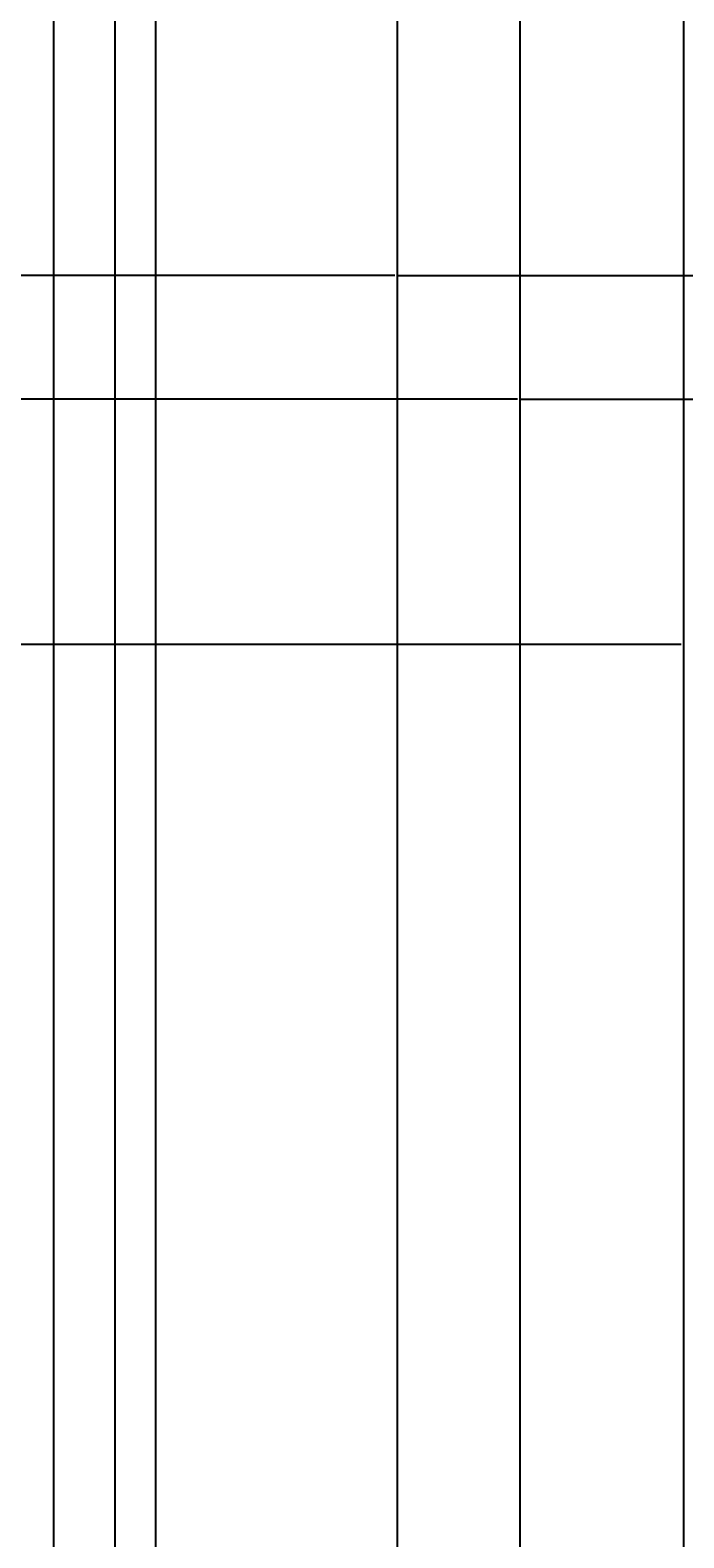
# Model space of a CAD drawing. Units: inches. Extents: x -6 to 289, y -8 to 323.
# Tile 25 of 107: x 126 to 142, y 87 to 124. Entities that reach past the tile are written whole.
import ezdxf

# ---------------------------------------------------------------- set-up
doc = ezdxf.new("R2010")
doc.units = ezdxf.units.IN
doc.header["$MEASUREMENT"] = 0
doc.layers.add('A-ANNO-DIMS', color=2, linetype='Continuous', lineweight=18)
doc.layers.add('A-DOOR', color=3, linetype='Continuous', lineweight=25)
doc.styles.get("Standard").update_dxf_attribs({"font": 'arial.ttf'})
doc.dimstyles.get("Standard").update_dxf_attribs({"dimtxt": 0.18, "dimasz": 0.18, "dimexe": 0.18, "dimexo": 0.0625, "dimgap": 0.09, "dimtad": 0, "dimtih": 1, "dimtoh": 1, "dimdec": 4, "dimzin": 0, "dimdsep": 46, "dimtxsty": 'Standard', "dimcen": 0.09, "dimadec": 0, "dimazin": 0, "dimtfac": 1, "dimtdec": 4, "dimtofl": 0, "dimtmove": 0, "dimatfit": 3, "dimfxl": 1, "dimtolj": 1, "dimtzin": 0, "dimarcsym": 0})

# ---------------------------------------------------------------- blocks, each defined once
blk = doc.blocks.new('*D28')
at = {"layer": 'A-ANNO-DIMS', "color": 0, "lineweight": -2, "transparency": 16777216}
for p, q in [((128.383, 180.092), (128.383, -8.391)), ((126.883, 178.592), (126.883, -8.391)), ((127.063, -8.211), (127.387, -8.211)), ((128.203, -8.211), (127.88, -8.211))]:
    blk.add_line(p, q, dxfattribs=at)
at = {"layer": 'A-ANNO-DIMS', "color": 0, "transparency": 16777216}
for points in [[(127.063, -8.181), (127.063, -8.241), (126.883, -8.211)], [(128.203, -8.181), (128.203, -8.241), (128.383, -8.211)]]:
    blk.add_solid(points, dxfattribs=at)
at = {"layer": 'Defpoints', "color": 0, "transparency": 16777216}
for p in [(128.383, 180.154), (126.883, 178.654), (128.383, -8.211)]:
    blk.add_point(p, dxfattribs=at)
at = {"layer": 'A-ANNO-DIMS', "color": 0, "transparency": 16777216, "insert": (127.633, -8.211), "char_height": 0.18, "attachment_point": 5}
blk.add_mtext('\\A1;1.5', dxfattribs=at)
blk = doc.blocks.new('*D29')
at = {"layer": 'A-ANNO-DIMS', "color": 0, "lineweight": -2, "transparency": 16777216}
for p, q in [((129.383, 181.092), (129.383, -8.391)), ((128.383, 180.092), (128.383, -8.391)), ((128.563, -8.211), (128.76, -8.211)), ((129.203, -8.211), (129.007, -8.211))]:
    blk.add_line(p, q, dxfattribs=at)
at = {"layer": 'A-ANNO-DIMS', "color": 0, "transparency": 16777216}
for points in [[(128.563, -8.181), (128.563, -8.241), (128.383, -8.211)], [(129.203, -8.181), (129.203, -8.241), (129.383, -8.211)]]:
    blk.add_solid(points, dxfattribs=at)
at = {"layer": 'Defpoints', "color": 0, "transparency": 16777216}
for p in [(129.383, 181.154), (128.383, 180.154), (129.383, -8.211)]:
    blk.add_point(p, dxfattribs=at)
at = {"layer": 'A-ANNO-DIMS', "color": 0, "transparency": 16777216, "insert": (128.883, -8.211), "char_height": 0.18, "attachment_point": 5}
blk.add_mtext('\\A1;1', dxfattribs=at)
blk = doc.blocks.new('*D30')
at = {"layer": 'A-ANNO-DIMS', "color": 0, "lineweight": -2, "transparency": 16777216}
for p, q in [((129.383, 181.092), (129.383, -8.391)), ((146.883, 181.092), (146.883, -8.391)), ((129.563, -8.211), (137.817, -8.211)), ((146.703, -8.211), (138.449, -8.211))]:
    blk.add_line(p, q, dxfattribs=at)
at = {"layer": 'A-ANNO-DIMS', "color": 0, "transparency": 16777216}
for points in [[(129.563, -8.181), (129.563, -8.241), (129.383, -8.211)], [(146.703, -8.181), (146.703, -8.241), (146.883, -8.211)]]:
    blk.add_solid(points, dxfattribs=at)
at = {"layer": 'Defpoints', "color": 0, "transparency": 16777216}
for p in [(129.383, 181.154), (146.883, 181.154), (146.883, -8.211)]:
    blk.add_point(p, dxfattribs=at)
at = {"layer": 'A-ANNO-DIMS', "color": 0, "transparency": 16777216, "insert": (138.133, -8.211), "char_height": 0.18, "attachment_point": 5}
blk.add_mtext('\\A1;17.5', dxfattribs=at)
blk = doc.blocks.new('*D73')
at = {"layer": 'A-ANNO-DIMS', "color": 0, "lineweight": -2, "transparency": 16777216}
for p, q in [((121.008, 51.148), (121.008, 322.969)), ((121.188, 322.789), (127.697, 322.789)), ((135.116, 322.789), (128.607, 322.789)), ((135.296, 51.148), (135.296, 322.969))]:
    blk.add_line(p, q, dxfattribs=at)
at = {"layer": 'A-ANNO-DIMS', "color": 0, "transparency": 16777216}
for points in [[(121.188, 322.819), (121.188, 322.759), (121.008, 322.789)], [(135.116, 322.819), (135.116, 322.759), (135.296, 322.789)]]:
    blk.add_solid(points, dxfattribs=at)
at = {"layer": 'Defpoints', "color": 0, "transparency": 16777216}
for p in [(135.296, 322.789), (121.008, 51.085), (135.296, 51.085)]:
    blk.add_point(p, dxfattribs=at)
at = {"layer": 'A-ANNO-DIMS', "color": 0, "transparency": 16777216, "insert": (128.152, 322.789), "char_height": 0.18, "attachment_point": 5}
blk.add_mtext('\\A1;14.288', dxfattribs=at)
blk = doc.blocks.new('*D74')
at = {"layer": 'A-ANNO-DIMS', "color": 0, "lineweight": -2, "transparency": 16777216}
for p, q in [((135.296, 51.148), (135.296, 322.969)), ((135.476, 322.789), (136.647, 322.789)), ((138.116, 322.789), (136.945, 322.789)), ((138.296, 51.148), (138.296, 322.969))]:
    blk.add_line(p, q, dxfattribs=at)
at = {"layer": 'A-ANNO-DIMS', "color": 0, "transparency": 16777216}
for points in [[(135.476, 322.819), (135.476, 322.759), (135.296, 322.789)], [(138.116, 322.819), (138.116, 322.759), (138.296, 322.789)]]:
    blk.add_solid(points, dxfattribs=at)
at = {"layer": 'Defpoints', "color": 0, "transparency": 16777216}
for p in [(138.296, 322.789), (135.296, 51.085), (138.296, 51.085)]:
    blk.add_point(p, dxfattribs=at)
at = {"layer": 'A-ANNO-DIMS', "color": 0, "transparency": 16777216, "insert": (136.796, 322.789), "char_height": 0.18, "attachment_point": 5}
blk.add_mtext('\\A1;3', dxfattribs=at)
blk = doc.blocks.new('*D75')
at = {"layer": 'A-ANNO-DIMS', "color": 0, "lineweight": -2, "transparency": 16777216}
for p, q in [((138.296, 51.148), (138.296, 322.969)), ((138.476, 322.789), (140.144, 322.789)), ((142.116, 322.789), (140.448, 322.789)), ((142.296, 51.148), (142.296, 322.969))]:
    blk.add_line(p, q, dxfattribs=at)
at = {"layer": 'A-ANNO-DIMS', "color": 0, "transparency": 16777216}
for points in [[(138.476, 322.819), (138.476, 322.759), (138.296, 322.789)], [(142.116, 322.819), (142.116, 322.759), (142.296, 322.789)]]:
    blk.add_solid(points, dxfattribs=at)
at = {"layer": 'Defpoints', "color": 0, "transparency": 16777216}
for p in [(142.296, 322.789), (138.296, 51.085), (142.296, 51.085)]:
    blk.add_point(p, dxfattribs=at)
at = {"layer": 'A-ANNO-DIMS', "color": 0, "transparency": 16777216, "insert": (140.296, 322.789), "char_height": 0.18, "attachment_point": 5}
blk.add_mtext('\\A1;4', dxfattribs=at)
blk = doc.blocks.new('*D76')
at = {"layer": 'A-ANNO-DIMS', "color": 0, "lineweight": -2, "transparency": 16777216}
for p, q in [((142.296, 51.148), (142.296, 322.969)), ((142.476, 322.789), (153.076, 322.789)), ((164.116, 322.789), (153.516, 322.789)), ((164.296, 51.148), (164.296, 322.969))]:
    blk.add_line(p, q, dxfattribs=at)
at = {"layer": 'A-ANNO-DIMS', "color": 0, "transparency": 16777216}
for points in [[(142.476, 322.819), (142.476, 322.759), (142.296, 322.789)], [(164.116, 322.819), (164.116, 322.759), (164.296, 322.789)]]:
    blk.add_solid(points, dxfattribs=at)
at = {"layer": 'Defpoints', "color": 0, "transparency": 16777216}
for p in [(164.296, 322.789), (142.296, 51.085), (164.296, 51.085)]:
    blk.add_point(p, dxfattribs=at)
at = {"layer": 'A-ANNO-DIMS', "color": 0, "transparency": 16777216, "insert": (153.296, 322.789), "char_height": 0.18, "attachment_point": 5}
blk.add_mtext('\\A1;22', dxfattribs=at)
blk = doc.blocks.new('*D87')
at = {"layer": 'A-ANNO-DIMS', "color": 0, "lineweight": -2, "transparency": 16777216}
for p, q in [((142.233, 108.948), (-5.737, 108.948)), ((-5.557, 108.768), (-5.557, 92.641)), ((-5.557, 76.151), (-5.557, 92.277)), ((166.233, 75.971), (-5.737, 75.971))]:
    blk.add_line(p, q, dxfattribs=at)
at = {"layer": 'A-ANNO-DIMS', "color": 0, "transparency": 16777216}
for points in [[(-5.587, 108.768), (-5.527, 108.768), (-5.557, 108.948)], [(-5.587, 76.151), (-5.527, 76.151), (-5.557, 75.971)]]:
    blk.add_solid(points, dxfattribs=at)
at = {"layer": 'Defpoints', "color": 0, "transparency": 16777216}
for p in [(-5.557, 108.948), (142.296, 108.948), (166.296, 75.971)]:
    blk.add_point(p, dxfattribs=at)
at = {"layer": 'A-ANNO-DIMS', "color": 0, "transparency": 16777216, "insert": (-5.557, 92.459), "char_height": 0.18, "attachment_point": 5}
blk.add_mtext('\\A1;32.98', dxfattribs=at)
blk = doc.blocks.new('*D88')
at = {"layer": 'A-ANNO-DIMS', "color": 0, "lineweight": -2, "transparency": 16777216}
for p, q in [((138.233, 114.948), (-5.737, 114.948)), ((-5.557, 114.768), (-5.557, 112.13)), ((-5.557, 109.128), (-5.557, 111.766)), ((142.233, 108.948), (-5.737, 108.948))]:
    blk.add_line(p, q, dxfattribs=at)
at = {"layer": 'A-ANNO-DIMS', "color": 0, "transparency": 16777216}
for points in [[(-5.587, 114.768), (-5.527, 114.768), (-5.557, 114.948)], [(-5.587, 109.128), (-5.527, 109.128), (-5.557, 108.948)]]:
    blk.add_solid(points, dxfattribs=at)
at = {"layer": 'Defpoints', "color": 0, "transparency": 16777216}
for p in [(-5.557, 114.948), (138.296, 114.948), (142.296, 108.948)]:
    blk.add_point(p, dxfattribs=at)
at = {"layer": 'A-ANNO-DIMS', "color": 0, "transparency": 16777216, "insert": (-5.557, 111.948), "char_height": 0.18, "attachment_point": 5}
blk.add_mtext('\\A1;6', dxfattribs=at)
blk = doc.blocks.new('*D89')
at = {"layer": 'A-ANNO-DIMS', "color": 0, "lineweight": -2, "transparency": 16777216}
for p, q in [((135.233, 117.971), (-5.737, 117.971)), ((-5.557, 117.791), (-5.557, 116.641)), ((-5.557, 115.128), (-5.557, 116.277)), ((138.233, 114.948), (-5.737, 114.948))]:
    blk.add_line(p, q, dxfattribs=at)
at = {"layer": 'A-ANNO-DIMS', "color": 0, "transparency": 16777216}
for points in [[(-5.587, 117.791), (-5.527, 117.791), (-5.557, 117.971)], [(-5.587, 115.128), (-5.527, 115.128), (-5.557, 114.948)]]:
    blk.add_solid(points, dxfattribs=at)
at = {"layer": 'Defpoints', "color": 0, "transparency": 16777216}
for p in [(-5.557, 117.971), (135.296, 117.971), (138.296, 114.948)]:
    blk.add_point(p, dxfattribs=at)
at = {"layer": 'A-ANNO-DIMS', "color": 0, "transparency": 16777216, "insert": (-5.557, 116.459), "char_height": 0.18, "attachment_point": 5}
blk.add_mtext('\\A1;3.023', dxfattribs=at)

msp = doc.modelspace()

# ---------------------------------------------------------------- linework, layer by layer
at = {"layer": 'A-DOOR'}
for points in [[(135.296, 51.0851), (135.296, 117.9706), (171.296, 117.9706), (171.296, 51.0851)], [(138.296, 51.0851), (138.296, 114.9477), (168.296, 114.9477), (168.296, 51.0851)]]:
    msp.add_lwpolyline(points, dxfattribs=at)

# ---------------------------------------------------------------- dimensions: what is measured, and where the dimension line sits
at = {"layer": 'A-ANNO-DIMS'}
for base, p1, p2, override, picture, middle in [((135.296, 322.7888), (121.008, 51.0851), (135.296, 51.0851), {"dimdec": 3, "dimlfac": 1, "dimrnd": 0, "dimzin": 0, "dimdsep": 46, "dimlunit": 2}, '*D73', (128.152, 322.7888)), ((138.296, 322.7888), (135.296, 51.0851), (138.296, 51.0851), {"dimdec": 0, "dimlfac": 1, "dimrnd": 0, "dimzin": 0, "dimdsep": 46, "dimlunit": 2}, '*D74', (136.796, 322.7888)), ((142.296, 322.7888), (138.296, 51.0851), (142.296, 51.0851), {"dimdec": 0, "dimlfac": 1, "dimrnd": 0, "dimzin": 0, "dimdsep": 46, "dimlunit": 2}, '*D75', (140.296, 322.7888)), ((164.296, 322.7888), (142.296, 51.0851), (164.296, 51.0851), {"dimdec": 0, "dimlfac": 1, "dimrnd": 0, "dimzin": 0, "dimdsep": 46, "dimlunit": 2}, '*D76', (153.296, 322.7888)), ((129.3835, -8.2112), (128.3835, 180.154), (129.3835, 181.154), {"dimdec": 0, "dimlfac": 1, "dimrnd": 0, "dimzin": 0, "dimdsep": 46, "dimlunit": 2}, '*D29', (128.8835, -8.2112)), ((146.8835, -8.2112), (129.3835, 181.154), (146.8835, 181.154), {"dimdec": 1, "dimlfac": 1, "dimrnd": 0, "dimzin": 0, "dimdsep": 46, "dimlunit": 2}, '*D30', (138.1335, -8.2112)), ((128.3835, -8.2112), (126.8835, 178.654), (128.3835, 180.154), {"dimdec": 1, "dimlfac": 1, "dimrnd": 0, "dimzin": 0, "dimdsep": 46, "dimlunit": 2}, '*D28', (127.6335, -8.2112))]:
    dim = msp.add_linear_dim(base=base, p1=p1, p2=p2, dimstyle='Standard', override=override, dxfattribs=at)
    dim.commit()
    dim.dimension.update_dxf_attribs({"geometry": picture, "text_midpoint": middle})
for base, p1, p2, override, picture, middle in [((-5.557, 117.9706), (138.296, 114.9477), (135.296, 117.9706), {"dimdec": 3, "dimlfac": 1, "dimrnd": 0, "dimzin": 0, "dimdsep": 46, "dimlunit": 2}, '*D89', (-5.557, 116.4592)), ((-5.557, 114.9477), (142.296, 108.9477), (138.296, 114.9477), {"dimdec": 0, "dimlfac": 1, "dimrnd": 0, "dimzin": 0, "dimdsep": 46, "dimlunit": 2}, '*D88', (-5.557, 111.9477)), ((-5.557, 108.9477), (166.296, 75.9706), (142.296, 108.9477), {"dimdec": 2, "dimlfac": 1, "dimrnd": 0, "dimzin": 0, "dimdsep": 46, "dimlunit": 2}, '*D87', (-5.557, 92.4592))]:
    dim = msp.add_linear_dim(base=base, p1=p1, p2=p2, angle=90, dimstyle='Standard', override=override, dxfattribs=at)
    dim.commit()
    dim.dimension.update_dxf_attribs({"geometry": picture, "text_midpoint": middle})

doc.saveas('drawing.dxf')
